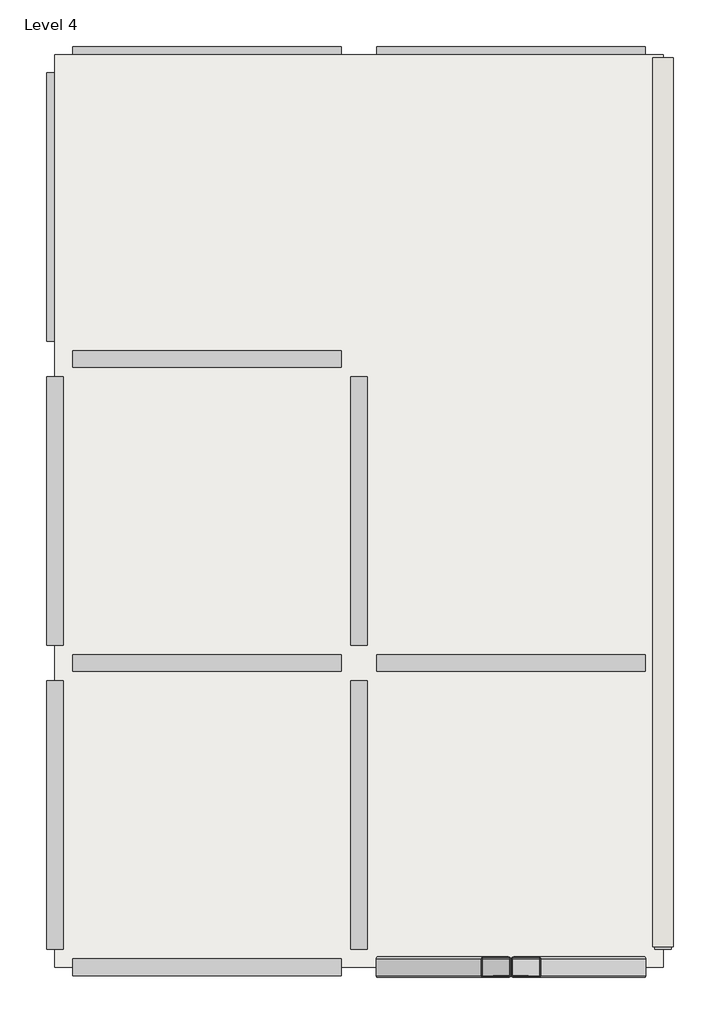
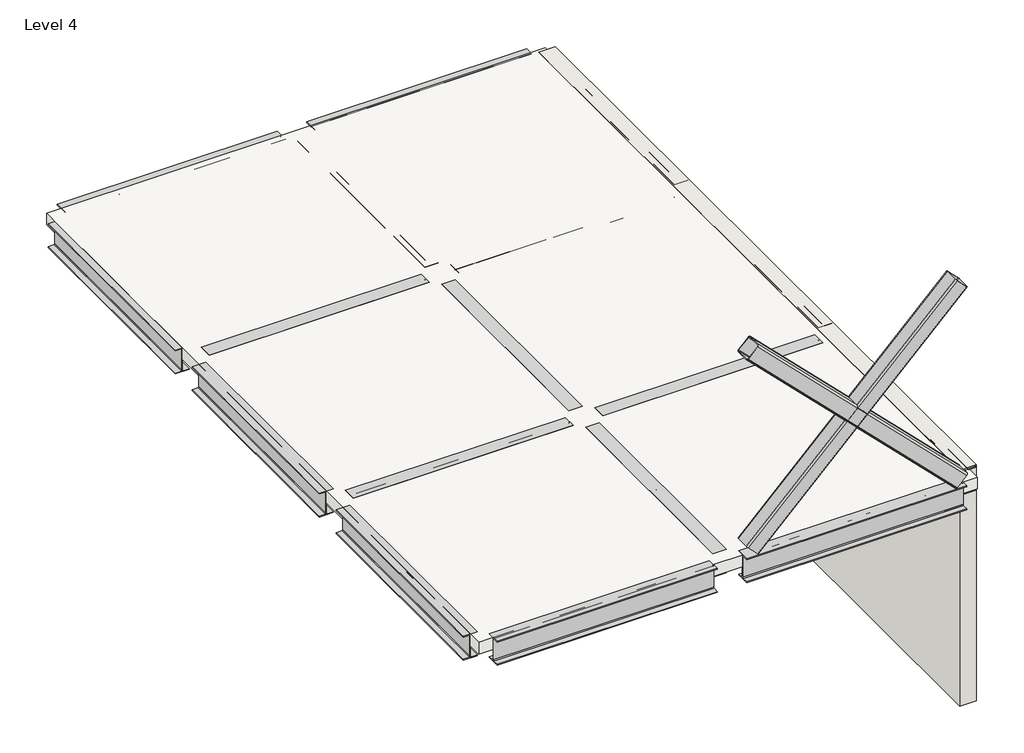
# One storey: 17 beams, 2 members, 1 slab, 1 wall.
"""IFC4 building model written with IfcOpenShell, lengths in millimetres."""

from ifc_helpers import new_model, si_unit, frame, origin, place, context, project, spatial, polyline, outline, extrude, transform, mapped, element, save
from components import ub_universal_beams_ub305x165x40_60ab2ee1, m_hss_square_hss203_2x203_2x9_5_07d005dd

model = new_model("IFC4")

# Units and contexts
model_context = context("Model", 3, world=origin())
ifc_project = project(units=[si_unit("LENGTHUNIT", "METRE", prefix="MILLI")], contexts=[model_context])

# Site, building, storey
site = spatial("IfcSite", under=ifc_project)
building = spatial("IfcBuilding", under=site)
storey = spatial("IfcBuildingStorey", under=building, Name="Level 4", Elevation=9000.0)

# Beams
placement = place(None, origin())
ub_universal_beams_ub305x165x40_shape = ub_universal_beams_ub305x165x40_60ab2ee1(model_context)
element("IfcBeam", 1, ObjectType="UB-Universal Beams : UB305x165x40", at=placement, inside=storey, context=model_context, shape_type="MappedRepresentation", body=[
    mapped(ub_universal_beams_ub305x165x40_shape, transform((18435.1404262, -6314.7314166, 8848.3), x_axis=(-1.0, 0.0, 0.0), y_axis=(0.0, -1.0, 0.0), z_axis=(0.0, 0.0, 1.0))),
])
element("IfcBeam", 2, ObjectType="UB-Universal Beams : UB305x165x40", at=placement, inside=storey, context=model_context, shape_type="MappedRepresentation", body=[
    mapped(ub_universal_beams_ub305x165x40_shape, transform((15435.1404262, -6314.7314166, 8848.3), x_axis=(-1.0, 0.0, 0.0), y_axis=(0.0, -1.0, 0.0), z_axis=(0.0, 0.0, 1.0))),
])
element("IfcBeam", 3, ObjectType="UB-Universal Beams : UB305x165x40", at=placement, inside=storey, context=model_context, shape_type="MappedRepresentation", body=[
    mapped(ub_universal_beams_ub305x165x40_shape, transform((13935.1404262, -4814.7314166, 8848.3), x_axis=(0.0, 1.0, 0.0), y_axis=(-1.0, 0.0, 0.0), z_axis=(0.0, 0.0, 1.0))),
])
element("IfcBeam", 4, ObjectType="UB-Universal Beams : UB305x165x40", at=placement, inside=storey, context=model_context, shape_type="MappedRepresentation", body=[
    mapped(ub_universal_beams_ub305x165x40_shape, transform((13935.1404262, -1814.7314166, 8848.3), x_axis=(0.0, 1.0, 0.0), y_axis=(-1.0, 0.0, 0.0), z_axis=(0.0, 0.0, 1.0))),
])
element("IfcBeam", 5, ObjectType="UB-Universal Beams : UB305x165x40", at=placement, inside=storey, context=model_context, shape_type="MappedRepresentation", body=[
    mapped(ub_universal_beams_ub305x165x40_shape, transform((13935.1404262, 1185.2685834, 8848.3), x_axis=(0.0, 1.0, 0.0), y_axis=(-1.0, 0.0, 0.0), z_axis=(0.0, 0.0, 1.0))),
])
element("IfcBeam", 6, ObjectType="UB-Universal Beams : UB305x165x40", at=placement, inside=storey, context=model_context, shape_type="MappedRepresentation", body=[
    mapped(ub_universal_beams_ub305x165x40_shape, transform((18435.1404262, -3314.7314166, 8848.3), x_axis=(-1.0, 0.0, 0.0), y_axis=(0.0, -1.0, 0.0), z_axis=(0.0, 0.0, 1.0))),
])
element("IfcBeam", 7, ObjectType="UB-Universal Beams : UB305x165x40", at=placement, inside=storey, context=model_context, shape_type="MappedRepresentation", body=[
    mapped(ub_universal_beams_ub305x165x40_shape, transform((15435.1404262, -3314.7314166, 8848.3), x_axis=(-1.0, 0.0, 0.0), y_axis=(0.0, -1.0, 0.0), z_axis=(0.0, 0.0, 1.0))),
])
element("IfcBeam", 8, ObjectType="UB-Universal Beams : UB305x165x40", at=placement, inside=storey, context=model_context, shape_type="MappedRepresentation", body=[
    mapped(ub_universal_beams_ub305x165x40_shape, transform((18435.1404262, -314.7314166, 8848.3), x_axis=(-1.0, 0.0, 0.0), y_axis=(0.0, -1.0, 0.0), z_axis=(0.0, 0.0, 1.0))),
])
element("IfcBeam", 9, ObjectType="UB-Universal Beams : UB305x165x40", at=placement, inside=storey, context=model_context, shape_type="MappedRepresentation", body=[
    mapped(ub_universal_beams_ub305x165x40_shape, transform((15435.1404262, -314.7314166, 8848.3), x_axis=(-1.0, 0.0, 0.0), y_axis=(0.0, -1.0, 0.0), z_axis=(0.0, 0.0, 1.0))),
])
element("IfcBeam", 10, ObjectType="UB-Universal Beams : UB305x165x40", at=placement, inside=storey, context=model_context, shape_type="MappedRepresentation", body=[
    mapped(ub_universal_beams_ub305x165x40_shape, transform((18435.1404262, 2685.2685834, 8848.3), x_axis=(-1.0, 0.0, 0.0), y_axis=(0.0, -1.0, 0.0), z_axis=(0.0, 0.0, 1.0))),
])
element("IfcBeam", 11, ObjectType="UB-Universal Beams : UB305x165x40", at=placement, inside=storey, context=model_context, shape_type="MappedRepresentation", body=[
    mapped(ub_universal_beams_ub305x165x40_shape, transform((15435.1404262, 2685.2685834, 8848.3), x_axis=(-1.0, 0.0, 0.0), y_axis=(0.0, -1.0, 0.0), z_axis=(0.0, 0.0, 1.0))),
])
element("IfcBeam", 12, ObjectType="UB-Universal Beams : UB305x165x40", at=placement, inside=storey, context=model_context, shape_type="MappedRepresentation", body=[
    mapped(ub_universal_beams_ub305x165x40_shape, transform((16935.1404262, -4814.7314166, 8848.3), x_axis=(0.0, 1.0, 0.0), y_axis=(-1.0, 0.0, 0.0), z_axis=(0.0, 0.0, 1.0))),
])
element("IfcBeam", 13, ObjectType="UB-Universal Beams : UB305x165x40", at=placement, inside=storey, context=model_context, shape_type="MappedRepresentation", body=[
    mapped(ub_universal_beams_ub305x165x40_shape, transform((16935.1404262, -1814.7314166, 8848.3), x_axis=(0.0, 1.0, 0.0), y_axis=(-1.0, 0.0, 0.0), z_axis=(0.0, 0.0, 1.0))),
])
element("IfcBeam", 14, ObjectType="UB-Universal Beams : UB305x165x40", at=placement, inside=storey, context=model_context, shape_type="MappedRepresentation", body=[
    mapped(ub_universal_beams_ub305x165x40_shape, transform((16935.1404262, 1185.2685834, 8848.3), x_axis=(0.0, 1.0, 0.0), y_axis=(-1.0, 0.0, 0.0), z_axis=(0.0, 0.0, 1.0))),
])
element("IfcBeam", 15, ObjectType="UB-Universal Beams : UB305x165x40", at=placement, inside=storey, context=model_context, shape_type="MappedRepresentation", body=[
    mapped(ub_universal_beams_ub305x165x40_shape, transform((19935.1404262, -1814.7314166, 8848.3), x_axis=(0.0, 1.0, 0.0), y_axis=(-1.0, 0.0, 0.0), z_axis=(0.0, 0.0, 1.0))),
])
element("IfcBeam", 16, ObjectType="UB-Universal Beams : UB305x165x40", at=placement, inside=storey, context=model_context, shape_type="MappedRepresentation", body=[
    mapped(ub_universal_beams_ub305x165x40_shape, transform((19935.1404262, 1185.2685834, 8848.3), x_axis=(0.0, 1.0, 0.0), y_axis=(-1.0, 0.0, 0.0), z_axis=(0.0, 0.0, 1.0))),
])
element("IfcBeam", 17, ObjectType="UB-Universal Beams : beam", at=placement, inside=storey, context=model_context, shape_type="MappedRepresentation", body=[
    mapped(ub_universal_beams_ub305x165x40_shape, transform((19935.1404262, -4814.7314166, 8848.3), x_axis=(0.0, 1.0, 0.0), y_axis=(-1.0, 0.0, 0.0), z_axis=(0.0, 0.0, 1.0))),
])

# Members
m_hss_square_hss203_2x203_2x9_5_shape = m_hss_square_hss203_2x203_2x9_5_07d005dd(model_context)
element("IfcMember", 18, ObjectType="M_HSS Square : HSS203.2X203.2X9.5", at=placement, inside=storey, context=model_context, shape_type="MappedRepresentation", body=[
    mapped(m_hss_square_hss203_2x203_2x9_5_shape, transform((18435.1404262, -6314.7314166, 10348.3), x_axis=(-0.7071067811865478, 0.0, 0.7071067811865476), y_axis=(0.0, -1.0000000000000002, 0.0), z_axis=(0.7071067811865476, 0.0, 0.7071067811865478))),
])
element("IfcMember", 19, ObjectType="M_HSS Square : HSS203.2X203.2X9.5", at=placement, inside=storey, context=model_context, shape_type="MappedRepresentation", body=[
    mapped(m_hss_square_hss203_2x203_2x9_5_shape, transform((18435.1404262, -6314.7314166, 10348.3), x_axis=(-0.7071067811865478, 0.0, -0.7071067811865475), y_axis=(0.0, -1.0000000000000002, 0.0), z_axis=(-0.7071067811865475, 0.0, 0.7071067811865478))),
])

# Slab
element("IfcSlab", 20, ObjectType="150mm Foundation Slab", at=placement, inside=storey, context=model_context, shape_type="SweptSolid", body=[
    extrude(outline(polyline([(13935.1404262, -6314.7314166), (13935.1404262, 2685.2685834), (19935.1404262, 2685.2685834), (19935.1404262, -6314.7314166), (13935.1404262, -6314.7314166)])), frame((0.0, 0.0, 8850.0), z_axis=(0.0, 0.0, 1.0), x_axis=(1.0, 0.0, 0.0)), (0.0, 0.0, 1.0), 150.0),
])

# Wall
element("IfcWall", 21, ObjectType="Generic - 200mm", at=placement, inside=storey, context=model_context, shape_type="SweptSolid", body=[
    extrude(outline(polyline([(19835.1404262, -6114.7314166), (19835.1404262, 2655.9792615), (20035.1404262, 2655.9792615), (20035.1404262, -6114.7314166), (19835.1404262, -6114.7314166)])), frame((0.0, 0.0, 6000.0), z_axis=(0.0, 0.0, 1.0), x_axis=(1.0, 0.0, 0.0)), (0.0, 0.0, 1.0), 3000.0),
])

save(model, "model.ifc")

# Revit data of these elements
# Type "UB-Universal Beams : UB305x165x40"
#   Section Name Key = "UB305X165X40"
#   Width = 16.5 cm
#   Web Thickness = 0.6 cm
#   Web Fillet = 0.89 cm
#   Warping Constant = 164000.0 cm⁶
#   Torsional Moment of Inertia = 14.70 cm⁴
#   Section Area = 51.3 cm²
#   Plastic Modulus weak axis = 142.0 cm³
#   Plastic Modulus strong axis = 623.0 cm³
#   Nominal Weight = 40.2999 kgf/m
#   Moment of Inertia weak axis = 764.00 cm⁴
#   Moment of Inertia strong axis = 8503.00 cm⁴
#   Height = 30.34 cm
#   Flange Thickness = 1.02 cm
#   Elastic Modulus weak axis = 92.6 cm³
#   Elastic Modulus strong axis = 560.0 cm³
#   Centroid Vertical = 15.17 cm
#   Centroid Horizontal = 8.25 cm
#   Bolt Spacing = 9.0 cm
#   Length [instance default] = 1.5 m
#   Structural Material [instance default] = Metal - Steel 43-275
#   Type Comments = ""
#   Assembly Code = ""
# Type "UB-Universal Beams : beam"
#   Section Name Key = "UB305X165X40"
#   Width = 16.5 cm
#   Web Thickness = 0.6 cm
#   Web Fillet = 0.89 cm
#   Warping Constant = 164000.0 cm⁶
#   Torsional Moment of Inertia = 14.70 cm⁴
#   Section Area = 51.3 cm²
#   Plastic Modulus weak axis = 142.0 cm³
#   Plastic Modulus strong axis = 623.0 cm³
#   Nominal Weight = 40.2999 kgf/m
#   Moment of Inertia weak axis = 764.00 cm⁴
#   Moment of Inertia strong axis = 8503.00 cm⁴
#   Height = 30.34 cm
#   Flange Thickness = 1.02 cm
#   Elastic Modulus weak axis = 92.6 cm³
#   Elastic Modulus strong axis = 560.0 cm³
#   Centroid Vertical = 15.17 cm
#   Centroid Horizontal = 8.25 cm
#   Bolt Spacing = 9.0 cm
#   Length [instance default] = 1.5 m
#   Structural Material [instance default] = Metal - Steel 43-275
#   Type Comments = ""
#   Assembly Code = ""
# Type "M_HSS Square : HSS203.2X203.2X9.5"
#   Section Name Key = "HSS 8X8X3/8"
#   Width = 20.3 cm
#   Wall Nominal Thickness = 0.953 cm
#   Wall Design Thickness = 0.886 cm
#   Torsional Moment of Inertia = 6660.00 cm⁴
#   Torsional Modulus = 10930171.7 cm³
#   Section Area = 67.1 cm²
#   Plastic Modulus weak axis = 482.0 cm³
#   Plastic Modulus strong axis = 482.0 cm³
#   Outer Fillet = 1.906 cm
#   Nominal Weight = 55.9998 kgf/m
#   Moment of Inertia weak axis = 4160.00 cm⁴
#   Moment of Inertia strong axis = 4160.00 cm⁴
#   Length [instance default] = 1.524 m
#   Inner Fillet = 0.953 cm
#   Height = 20.3 cm
#   Elastic Modulus weak axis = 408.0 cm³
#   Elastic Modulus strong axis = 408.0 cm³
#   Centroid Vertical = 10.15 cm
#   Centroid Horizontal = 10.15 cm
#   Structural Material [instance default] = Steel, 45-345
# Type "150mm Foundation Slab"
#   Layers, outside or top first: 0.15 m "Concrete, Cast-in-Place gray" (function 1)
# Type "Generic - 200mm"
#   Layers, outside or top first: 0.2 m no material (function 1)
# Elements 1, 2, 3, 4, 5, 6, 7, 8, 9, 10, 11, 12, 13, 14, 15, 16 (IfcBeam, "UB-Universal Beams : UB305x165x40")
#   Structural Material = Metal - Steel 43-275
#   Phase Created = New Construction
#   Materials on its faces: "Metal - Steel 43-275"
# Element 17 (IfcBeam, "UB-Universal Beams : beam")
#   Structural Material = Metal - Steel 43-275
#   Phase Created = New Construction
#   Materials on its faces: "Metal - Steel 43-275"
# Elements 18, 19 (IfcMember, "M_HSS Square : HSS203.2X203.2X9.5")
#   Comments = ""
#   Structural Material = Metal - Steel 43-275
#   Phase Created = New Construction
#   Materials on its faces: "Metal - Steel 43-275"
# Element 20 (IfcSlab, "150mm Foundation Slab")
#   built-in parameter 1001955 = 3.14159 (stored number, unit not read)
#   Height Offset From Level = 0 m
#   built-in parameter 1001954 = 1
#   Phase Created = New Construction
#   Materials on its faces: "Concrete, Cast-in-Place gray"
# Element 21 (IfcWall, "Generic - 200mm")
#   Comments = ""
#   built-in parameter 1001111 = -3 m
#   Top Offset = 0 m
#   Base Offset = -3 m
#   wall height = 3 m
#   Phase Created = New Construction
#   Base Constraint = Level 4
#   Top Constraint = Level 4
#   Materials on its faces: "Default Wall"
# Materials
#   "Metal - Steel 43-275": class "Metal", colour RGB 247 247 247, transparency 0, Cost = 0
#   "Steel, 45-345": class "Metal", colour RGB 247 247 247, transparency 0, Description = "Steel 345 MPa", Cost = 0
#   "Concrete, Cast-in-Place gray": class "Concrete", colour RGB 192 192 192, transparency 0, Description = "Cast-in-place concrete", Cost = 0
#   "Default Wall": colour RGB 128 128 128, transparency 0, Cost = 0
